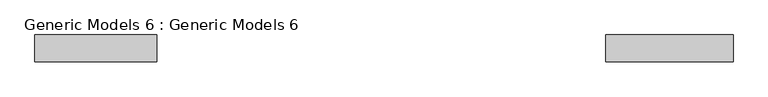
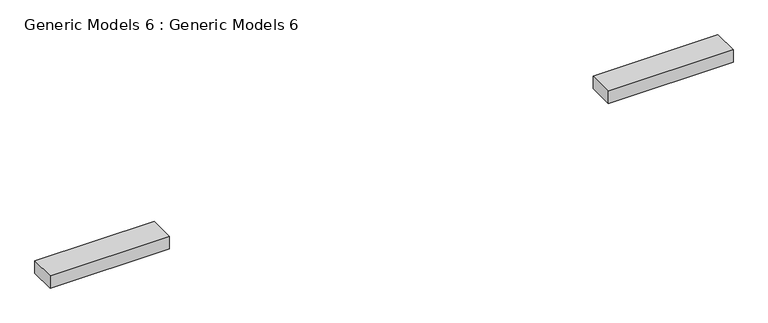
"""IFC4 building model written with IfcOpenShell, lengths in millimetres: proxy geometry, Generic Models 6 : Generic Models 6."""

from ifc_helpers import new_model, si_unit, frame, origin, place, context, project, spatial, polyline, outline, extrude, source, transform, mapped, element, save


def generic_models_6_generic_models_6_966f38bf(model_context):
    return source(origin(), model_context, "Body", "SweptSolid", [
        extrude(outline(polyline([(-13584.9655727, 7039.4500875), (-12199.3157907, 7039.4500875), (-12199.3157907, 6734.6500875), (-13584.9655727, 6734.6500875), (-13584.9655727, 7039.4500875)])), frame((0.0, 0.0, 2133.6), z_axis=(0.0, 0.0, 1.0), x_axis=(1.0, 0.0, 0.0)), (0.0, 0.0, 1.0), 152.4),
        extrude(outline(polyline([(-7094.3452422, 7039.4500875), (-5643.3621693, 7039.4500875), (-5643.3621693, 6734.6500875), (-7094.3452422, 6734.6500875), (-7094.3452422, 7039.4500875)])), frame((0.0, 0.0, 2133.6), z_axis=(0.0, 0.0, 1.0), x_axis=(1.0, 0.0, 0.0)), (0.0, 0.0, 1.0), 152.4),
    ])


if __name__ == "__main__":
    model = new_model("IFC4")
    model_context = context("Model", 3, world=origin())
    ifc_project = project(units=[si_unit("LENGTHUNIT", "METRE", prefix="MILLI")], contexts=[model_context])
    site = spatial("IfcSite", under=ifc_project)
    building = spatial("IfcBuilding", under=site)
    placement = place(None, origin())
    generic_models_6_generic_models_6_shape = generic_models_6_generic_models_6_966f38bf(model_context)
    element("IfcBuildingElementProxy", 1, Name="Generic Models 6 : Generic Models 6", ObjectType="Generic Models 6 : Generic Models 6", at=placement, inside=building, context=model_context, shape_type="MappedRepresentation", body=[
        mapped(generic_models_6_generic_models_6_shape, transform((0.0, 0.0, 0.0), x_axis=(1.0, 0.0, 0.0), y_axis=(0.0, 1.0, 0.0), z_axis=(0.0, 0.0, 1.0))),
    ])
    save(model, "model.ifc")

# Revit data of these elements
# Element 1 (IfcBuildingElementProxy, "Generic Models 6 : Generic Models 6")
#   Materials on its faces: "LIGHT BEIGE"
# Materials
#   "LIGHT BEIGE": class "Generic", colour RGB 120 120 120, transparency 0, Cost = 0
